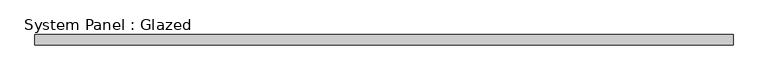
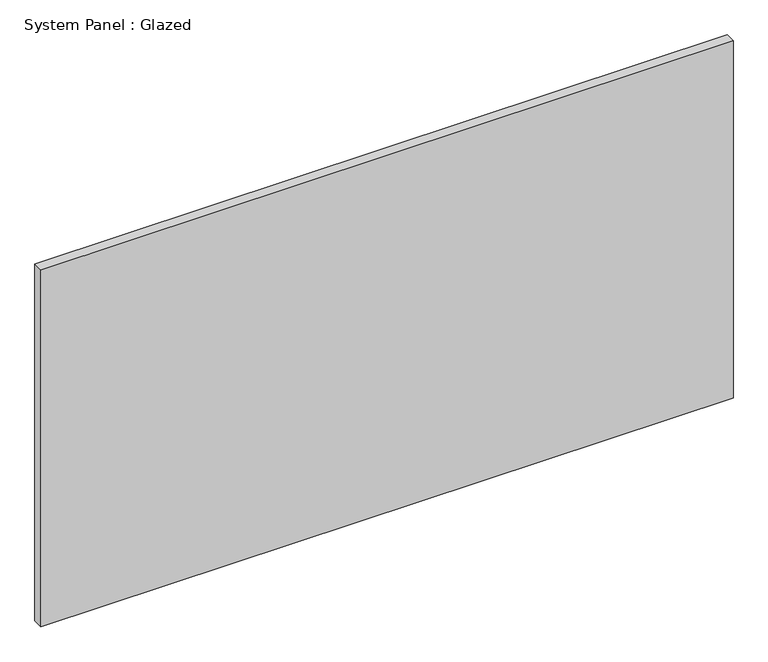
"""IFC4 building model written with IfcOpenShell, lengths in millimetres: plate geometry, System Panel : Glazed."""

from ifc_helpers import new_model, si_unit, origin, origin_with_axes, place, context, project, spatial, polyline, outline, extrude, source, transform, mapped, element, save


def system_panel_glazed_7be091cd(model_context):
    return source(origin(), model_context, "Body", "SweptSolid", [
        extrude(outline(polyline([(838.2, 19.05), (-838.2, 19.05), (-838.2, 44.45), (838.2, 44.45), (838.2, 19.05)])), origin_with_axes(), (0.0, 0.0, 1.0), 914.4),
    ])


if __name__ == "__main__":
    model = new_model("IFC4")
    model_context = context("Model", 3, world=origin())
    ifc_project = project(units=[si_unit("LENGTHUNIT", "METRE", prefix="MILLI")], contexts=[model_context])
    site = spatial("IfcSite", under=ifc_project)
    building = spatial("IfcBuilding", under=site)
    placement = place(None, origin())
    system_panel_glazed_shape = system_panel_glazed_7be091cd(model_context)
    element("IfcPlate", 1, ObjectType="System Panel : Glazed", at=placement, inside=building, context=model_context, shape_type="MappedRepresentation", body=[
        mapped(system_panel_glazed_shape, transform((0.0, 0.0, 0.0), x_axis=(1.0, 0.0, 0.0), y_axis=(0.0, 1.0, 0.0), z_axis=(0.0, 0.0, 1.0))),
    ])
    save(model, "model.ifc")

# Revit data of these elements
# Type "System Panel : Glazed"
#   Construction Type Id = "GSP4R"
#   Analytic Construction = "1/8 in Pilkington single glazing"
#   Visual Light Transmittance = 0.9
#   Solar Heat Gain Coefficient = 0.86
#   Heat Transfer Coefficient (U) = 6.7069 W/(m²·K)
# Element 1 (IfcPlate, "System Panel : Glazed")
#   Materials on its faces: "Glass"
# Materials
#   "Glass": class "Glass", colour RGB 0 128 192, transparency 0.75, Description = "Soda Lime Glass", Cost = 0
